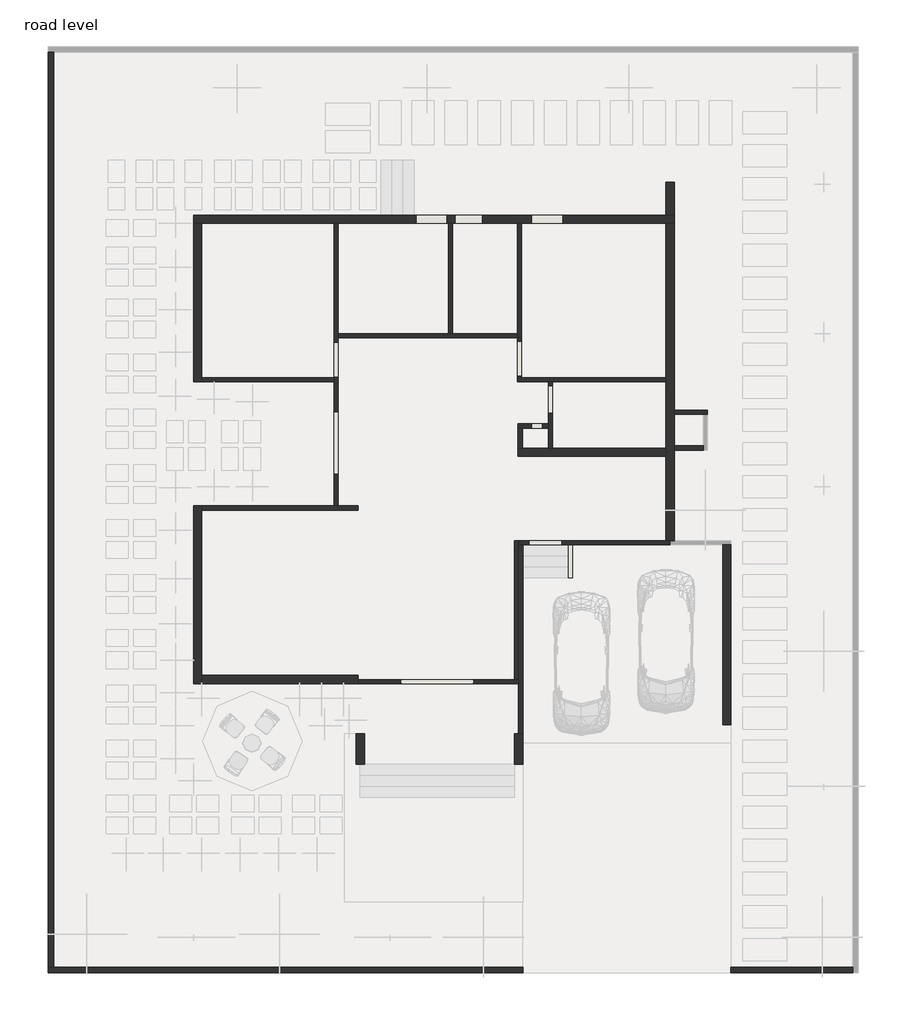
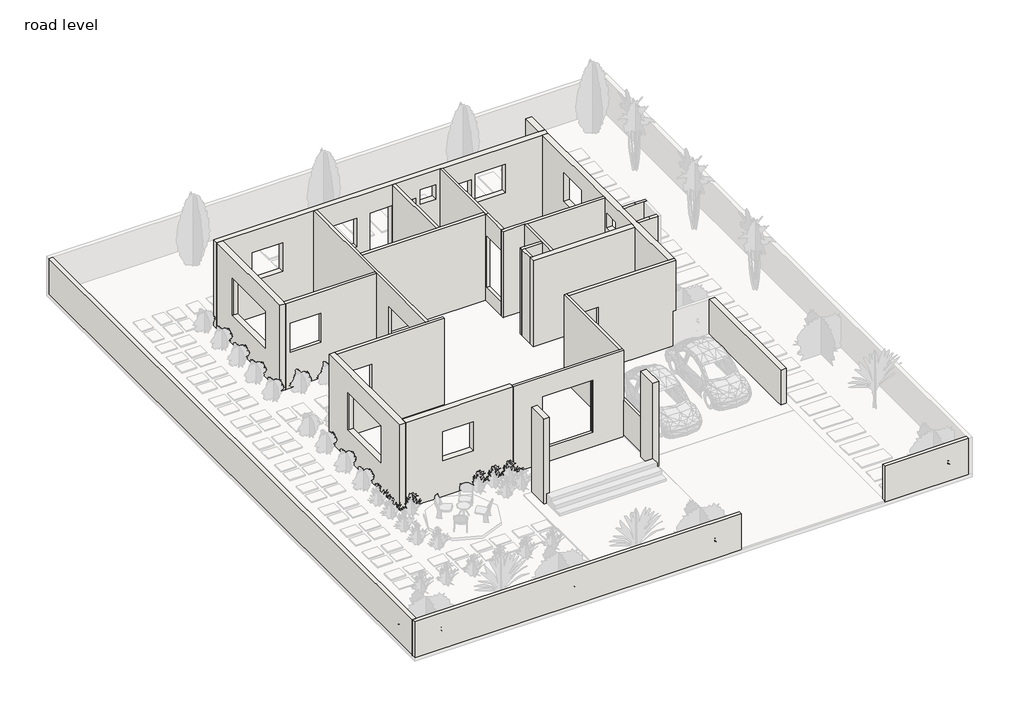
# One storey, part 1 of 3: 31 walls.
"""IFC4 building model written with IfcOpenShell, lengths in millimetres."""

from ifc_helpers import new_model, si_unit, frame, origin, origin_with_axes, place, context, project, spatial, polyline, outline, extrude, faceted_brep, element, save

model = new_model("IFC4")

# Units and contexts
model_context = context("Model", 3, world=origin())
ifc_project = project(units=[si_unit("LENGTHUNIT", "METRE", prefix="MILLI")], contexts=[model_context])

# Site, building, storey
site = spatial("IfcSite", under=ifc_project)
building = spatial("IfcBuilding", under=site)
storey = spatial("IfcBuildingStorey", under=building, Name="road level", Elevation=0.0)

# Walls
placement = place(None, origin())
element("IfcWall", 1, ObjectType="Generic - 4.5\"", at=placement, inside=storey, context=model_context, shape_type="Brep", body=[
    faceted_brep([(-10099.9719122, 10368.3168074, 0.0), (-10099.9719122, 6101.1168074, 0.0), (-10099.9719122, 5986.8168074, 0.0), (-10099.9719122, 2557.8168074, 0.0), (-10099.9719122, 2557.8168074, 3657.6), (-10099.9719122, 5986.8168074, 3657.6), (-10099.9719122, 6101.1168074, 3657.6), (-10099.9719122, 10368.3168074, 3657.6), (-10099.9719122, 6120.1668074, 609.6), (-10099.9719122, 7085.3668074, 609.6), (-10099.9719122, 7085.3668074, 2768.6), (-10099.9719122, 6120.1668074, 2768.6), (-10099.9719122, 5154.9668074, 2743.2), (-10099.9719122, 3427.7668074, 2743.2), (-10099.9719122, 3427.7668074, 609.6), (-10099.9719122, 5154.9668074, 609.6), (-9985.6719122, 10368.3168074, 0.0), (-9985.6719122, 10368.3168074, 3657.6), (-9985.6719122, 7320.3168074, 3657.6), (-9985.6719122, 7206.0168074, 3657.6), (-9985.6719122, 2557.8168074, 3657.6), (-9985.6719122, 2557.8168074, 0.0), (-9985.6719122, 7206.0168074, 0.0), (-9985.6719122, 7320.3168074, 0.0), (-9985.6719122, 6120.1668074, 609.6), (-9985.6719122, 6120.1668074, 2768.6), (-9985.6719122, 7085.3668074, 2768.6), (-9985.6719122, 7085.3668074, 609.6), (-9985.6719122, 5154.9668074, 2743.2), (-9985.6719122, 5154.9668074, 609.6), (-9985.6719122, 3427.7668074, 609.6), (-9985.6719122, 3427.7668074, 2743.2)], [[[0, 1, 2, 3, 4, 5, 6, 7], [8, 9, 10, 11], [12, 13, 14, 15]], [[16, 17, 18, 19, 20, 21, 22, 23], [24, 25, 26, 27], [28, 29, 30, 31]], [[3, 2, 1, 0, 16, 23, 22, 21]], [[0, 7, 17, 16]], [[4, 3, 21, 20]], [[25, 24, 8, 11]], [[26, 25, 11, 10]], [[27, 26, 10, 9]], [[24, 27, 9, 8]], [[29, 28, 12, 15]], [[30, 29, 15, 14]], [[31, 30, 14, 13]], [[28, 31, 13, 12]], [[7, 6, 5, 4, 20, 19, 18, 17]]]),
])
element("IfcWall", 2, ObjectType="Generic - 4.5\"", at=placement, inside=storey, context=model_context, shape_type="SweptSolid", body=[
    extrude(outline(polyline([(0.0, -10099.9719122), (3657.6, -10099.9719122), (3657.6, -13757.5719122), (0.0, -13757.5719122), (0.0, -10099.9719122)]), holes=[polyline([(2743.2, -13567.0719122), (2743.2, -12347.8719122), (1524.0, -12347.8719122), (1524.0, -13567.0719122), (2743.2, -13567.0719122)])]), frame((0.0, 5986.8168074, 0.0), z_axis=(0.0, 1.0, 0.0), x_axis=(0.0, 0.0, 1.0)), (0.0, 0.0, 1.0), 114.3),
])
element("IfcWall", 3, ObjectType="Generic - 4.5\"", at=placement, inside=storey, context=model_context, shape_type="Brep", body=[
    faceted_brep([(-5023.1469122, 10368.3168074, 0.0), (-5023.1469122, 7320.3168074, 0.0), (-5023.1469122, 7206.0168074, 0.0), (-5023.1469122, 7206.0168074, 3657.6), (-5023.1469122, 7320.3168074, 3657.6), (-5023.1469122, 10368.3168074, 3657.6), (-4908.8469122, 10368.3168074, 0.0), (-4908.8469122, 10368.3168074, 3657.6), (-4908.8469122, 7206.0168074, 3657.6), (-4908.8469122, 7206.0168074, 0.0)], [[[0, 1, 2, 3, 4, 5]], [[6, 7, 8, 9]], [[2, 1, 0, 6, 9]], [[0, 5, 7, 6]], [[3, 2, 9, 8]], [[5, 4, 3, 8, 7]]]),
])
element("IfcWall", 4, ObjectType="Generic - 4.5\"", at=placement, inside=storey, context=model_context, shape_type="Brep", body=[
    faceted_brep([(-5023.1469122, 7320.3168074, 0.0), (-6823.3719122, 7320.3168074, 0.0), (-6937.6719122, 7320.3168074, 0.0), (-9985.6719122, 7320.3168074, 0.0), (-9985.6719122, 7320.3168074, 3657.6), (-6937.6719122, 7320.3168074, 3657.6), (-6823.3719122, 7320.3168074, 3657.6), (-5023.1469122, 7320.3168074, 3657.6), (-5023.1469122, 7206.0168074, 0.0), (-5023.1469122, 7206.0168074, 3657.6), (-9985.6719122, 7206.0168074, 3657.6), (-9985.6719122, 7206.0168074, 0.0)], [[[0, 1, 2, 3, 4, 5, 6, 7]], [[8, 9, 10, 11]], [[3, 2, 1, 0, 8, 11]], [[0, 7, 9, 8]], [[4, 3, 11, 10]], [[7, 6, 5, 4, 10, 9]]]),
])
element("IfcWall", 5, ObjectType="Generic - 4.5\"", at=placement, inside=storey, context=model_context, shape_type="SweptSolid", body=[
    extrude(outline(polyline([(-6937.6719122, 7320.3168074), (-6937.6719122, 10368.3168074), (-6823.3719122, 10368.3168074), (-6823.3719122, 7320.3168074), (-6937.6719122, 7320.3168074)])), origin_with_axes(), (0.0, 0.0, 1.0), 3657.6),
])
element("IfcWall", 6, ObjectType="Generic - 4.5\"", at=placement, inside=storey, context=model_context, shape_type="Brep", body=[
    faceted_brep([(-917.8719122, 6101.1168074, 0.0), (-4908.8469122, 6101.1168074, 0.0), (-5023.1469122, 6101.1168074, 0.0), (-5023.1469122, 6101.1168074, 3657.6), (-4908.8469122, 6101.1168074, 3657.6), (-917.8719122, 6101.1168074, 3657.6), (-917.8719122, 5986.8168074, 0.0), (-917.8719122, 5986.8168074, 3657.6), (-4054.7719122, 5986.8168074, 3657.6), (-4169.0719122, 5986.8168074, 3657.6), (-5023.1469122, 5986.8168074, 3657.6), (-5023.1469122, 5986.8168074, 0.0), (-4169.0719122, 5986.8168074, 0.0), (-4054.7719122, 5986.8168074, 0.0)], [[[0, 1, 2, 3, 4, 5]], [[6, 7, 8, 9, 10, 11, 12, 13]], [[2, 1, 0, 6, 13, 12, 11]], [[3, 2, 11, 10]], [[0, 5, 7, 6]], [[5, 4, 3, 10, 9, 8, 7]]]),
])
element("IfcWall", 7, ObjectType="Generic - 4.5\"", at=placement, inside=storey, context=model_context, shape_type="SweptSolid", body=[
    extrude(outline(polyline([(6101.1168074, 0.0), (6101.1168074, 3657.6), (7206.0168074, 3657.6), (7206.0168074, 0.0), (6101.1168074, 0.0)]), holes=[polyline([(6142.3918074, 609.6), (7107.5918074, 609.6), (7107.5918074, 2768.6), (6142.3918074, 2768.6), (6142.3918074, 609.6)])]), frame((-5023.1469122, 0.0, 0.0), z_axis=(1.0, 0.0, 0.0), x_axis=(0.0, 1.0, 0.0)), (0.0, 0.0, 1.0), 114.3),
])
element("IfcWall", 8, ObjectType="Generic - 4.5\"", at=placement, inside=storey, context=model_context, shape_type="Brep", body=[
    faceted_brep([(-13757.5719122, 2443.5168074, 0.0), (-9433.2219122, 2443.5168074, 0.0), (-9433.2219122, 2443.5168074, 3657.6), (-13757.5719122, 2443.5168074, 3657.6), (-12347.8719122, 2443.5168074, 2743.2), (-12347.8719122, 2443.5168074, 1524.0), (-13567.0719122, 2443.5168074, 1524.0), (-13567.0719122, 2443.5168074, 2743.2), (-13757.5719122, 2557.8168074, 0.0), (-13757.5719122, 2557.8168074, 3657.6), (-10099.9719122, 2557.8168074, 3657.6), (-9985.6719122, 2557.8168074, 3657.6), (-9433.2219122, 2557.8168074, 3657.6), (-9433.2219122, 2557.8168074, 0.0), (-9985.6719122, 2557.8168074, 0.0), (-10099.9719122, 2557.8168074, 0.0), (-12347.8719122, 2557.8168074, 2743.2), (-13567.0719122, 2557.8168074, 2743.2), (-13567.0719122, 2557.8168074, 1524.0), (-12347.8719122, 2557.8168074, 1524.0)], [[[0, 1, 2, 3], [4, 5, 6, 7]], [[8, 9, 10, 11, 12, 13, 14, 15], [16, 17, 18, 19]], [[1, 0, 8, 15, 14, 13]], [[2, 1, 13, 12]], [[0, 3, 9, 8]], [[5, 4, 16, 19]], [[6, 5, 19, 18]], [[7, 6, 18, 17]], [[4, 7, 17, 16]], [[3, 2, 12, 11, 10, 9]]]),
])
element("IfcWall", 9, ObjectType="Generic - 4.5\"", at=placement, inside=storey, context=model_context, shape_type="Brep", body=[
    faceted_brep([(-9433.2219122, -2357.0831926, 0.0), (-4994.5719122, -2357.0831926, 0.0), (-4994.5719122, -2357.0831926, 3657.6), (-9433.2219122, -2357.0831926, 3657.6), (-8242.4719122, -2357.0831926, 2818.6), (-6242.4719122, -2357.0831926, 2818.6), (-6242.4719122, -2357.0831926, 609.6), (-8242.4719122, -2357.0831926, 609.6), (-4994.5719122, -2242.7831926, 0.0), (-5108.8719122, -2242.7831926, 0.0), (-9433.2219122, -2242.7831926, 0.0), (-9433.2219122, -2242.7831926, 3657.6), (-5108.8719122, -2242.7831926, 3657.6), (-4994.5719122, -2242.7831926, 3657.6), (-6242.4719122, -2242.7831926, 2818.6), (-8242.4719122, -2242.7831926, 2818.6), (-8242.4719122, -2242.7831926, 609.6), (-6242.4719122, -2242.7831926, 609.6), (-6242.4719122, -2262.7831926, 2818.6), (-8242.4719122, -2262.7831926, 2818.6), (-8242.4719122, -2332.7831926, 2818.6), (-6242.4719122, -2332.7831926, 2818.6), (-6242.4719122, -2332.7831926, 609.6), (-6227.4719122, -2332.7831926, 609.6), (-6227.4719122, -2262.7831926, 609.6), (-6242.4719122, -2262.7831926, 609.6), (-8242.4719122, -2262.7831926, 609.6), (-8257.4719122, -2262.7831926, 609.6), (-8257.4719122, -2332.7831926, 609.6), (-8242.4719122, -2332.7831926, 609.6), (-8257.4719122, -2332.7831926, 2833.6), (-6227.4719122, -2332.7831926, 2833.6), (-6227.4719122, -2262.7831926, 2833.6), (-8257.4719122, -2262.7831926, 2833.6)], [[[0, 1, 2, 3], [4, 5, 6, 7]], [[8, 9, 10, 11, 12, 13], [14, 15, 16, 17]], [[1, 0, 10, 9, 8]], [[0, 3, 11, 10]], [[2, 1, 8, 13]], [[18, 19, 15, 14]], [[20, 21, 5, 4]], [[22, 23, 24, 25, 17, 16, 26, 27, 28, 29, 7, 6]], [[29, 20, 4, 7]], [[21, 22, 6, 5]], [[21, 20, 29, 28, 30, 31, 23, 22]], [[24, 23, 31, 32]], [[19, 18, 25, 24, 32, 33, 27, 26]], [[25, 18, 14, 17]], [[19, 26, 16, 15]], [[28, 27, 33, 30]], [[31, 30, 33, 32]], [[3, 2, 13, 12, 11]]]),
])
element("IfcWall", 10, ObjectType="Generic - 4.5\"", at=placement, inside=storey, context=model_context, shape_type="Brep", body=[
    faceted_brep([(-4994.5719122, -2242.7831926, 0.0), (-4994.5719122, 1481.4918074, 0.0), (-4994.5719122, 1595.7918074, 0.0), (-4994.5719122, 1595.7918074, 3657.6), (-4994.5719122, 1481.4918074, 3657.6), (-4994.5719122, -2242.7831926, 3657.6), (-5108.8719122, -2242.7831926, 0.0), (-5108.8719122, -2242.7831926, 3657.6), (-5108.8719122, 1595.7918074, 3657.6), (-5108.8719122, 1595.7918074, 0.0)], [[[0, 1, 2, 3, 4, 5]], [[6, 7, 8, 9]], [[2, 1, 0, 6, 9]], [[0, 5, 7, 6]], [[3, 2, 9, 8]], [[5, 4, 3, 8, 7]]]),
])
element("IfcWall", 11, ObjectType="Generic - 4.5\"", at=placement, inside=storey, context=model_context, shape_type="Brep", body=[
    faceted_brep([(-4994.5719122, 1481.4918074, 0.0), (-4993.7781622, 1481.4918074, 0.0), (-4879.4781622, 1481.4918074, 0.0), (-3616.6219122, 1481.4918074, 0.0), (-3502.3219122, 1481.4918074, 0.0), (-803.5719122, 1481.4918074, 0.0), (-803.5719122, 1481.4918074, 1524.0), (-689.2719122, 1481.4918074, 1524.0), (-689.2719122, 1481.4918074, 3657.6), (-4994.5719122, 1481.4918074, 3657.6), (-4708.0281622, 1481.4918074, 2743.2), (-3793.6281622, 1481.4918074, 2743.2), (-3793.6281622, 1481.4918074, 609.6), (-4708.0281622, 1481.4918074, 609.6), (-4994.5719122, 1595.7918074, 0.0), (-4994.5719122, 1595.7918074, 3657.6), (-917.8719122, 1595.7918074, 3657.6), (-689.2719122, 1595.7918074, 3657.6), (-689.2719122, 1595.7918074, 1524.0), (-803.5719122, 1595.7918074, 1524.0), (-803.5719122, 1595.7918074, 0.0), (-917.8719122, 1595.7918074, 0.0), (-4708.0281622, 1595.7918074, 2743.2), (-4708.0281622, 1595.7918074, 609.6), (-3793.6281622, 1595.7918074, 609.6), (-3793.6281622, 1595.7918074, 2743.2)], [[[0, 1, 2, 3, 4, 5, 6, 7, 8, 9], [10, 11, 12, 13]], [[14, 15, 16, 17, 18, 19, 20, 21], [22, 23, 24, 25]], [[5, 4, 3, 2, 1, 0, 14, 21, 20]], [[0, 9, 15, 14]], [[6, 5, 20, 19]], [[18, 7, 6, 19]], [[8, 7, 18, 17]], [[23, 22, 10, 13]], [[24, 23, 13, 12]], [[25, 24, 12, 11]], [[22, 25, 11, 10]], [[9, 8, 17, 16, 15]]]),
])
element("IfcWall", 12, ObjectType="Generic - 4.5\"", at=placement, inside=storey, context=model_context, shape_type="SweptSolid", body=[
    extrude(outline(polyline([(-4879.4781622, 1481.4918074), (-4879.4781622, -3741.3831926), (-4993.7781622, -3741.3831926), (-4993.7781622, 1481.4918074), (-4879.4781622, 1481.4918074)])), origin_with_axes(), (0.0, 0.0, 1.0), 1524.0),
])
element("IfcWall", 13, ObjectType="Generic - 4.5\"", at=placement, inside=storey, context=model_context, shape_type="SweptSolid", body=[
    extrude(outline(polyline([(-3502.3219122, 1481.4918074), (-3502.3219122, 566.1722231), (-3616.6219122, 566.1722231), (-3616.6219122, 1481.4918074), (-3502.3219122, 1481.4918074)])), origin_with_axes(), (0.0, 0.0, 1.0), 609.6),
])
element("IfcWall", 14, ObjectType="Generic - 4.5\"", at=placement, inside=storey, context=model_context, shape_type="Brep", body=[
    faceted_brep([(-4054.7719122, 4158.0168074, 0.0), (-4054.7719122, 5986.8168074, 0.0), (-4054.7719122, 5986.8168074, 3657.6), (-4054.7719122, 4158.0168074, 3657.6), (-4054.7719122, 5123.2168074, 609.6), (-4054.7719122, 5123.2168074, 2743.2), (-4054.7719122, 5885.2168074, 2743.2), (-4054.7719122, 5885.2168074, 609.6), (-4169.0719122, 4158.0168074, 0.0), (-4169.0719122, 4158.0168074, 3657.6), (-4169.0719122, 4710.4668074, 3657.6), (-4169.0719122, 4824.7668074, 3657.6), (-4169.0719122, 5986.8168074, 3657.6), (-4169.0719122, 5986.8168074, 0.0), (-4169.0719122, 4824.7668074, 0.0), (-4169.0719122, 4710.4668074, 0.0), (-4169.0719122, 5123.2168074, 609.6), (-4169.0719122, 5885.2168074, 609.6), (-4169.0719122, 5885.2168074, 2743.2), (-4169.0719122, 5123.2168074, 2743.2)], [[[0, 1, 2, 3], [4, 5, 6, 7]], [[8, 9, 10, 11, 12, 13, 14, 15], [16, 17, 18, 19]], [[1, 0, 8, 15, 14, 13]], [[2, 1, 13, 12]], [[0, 3, 9, 8]], [[17, 16, 4, 7]], [[18, 17, 7, 6]], [[19, 18, 6, 5]], [[16, 19, 5, 4]], [[3, 2, 12, 11, 10, 9]]]),
])
element("IfcWall", 15, ObjectType="Generic - 4.5\"", at=placement, inside=storey, context=model_context, shape_type="SweptSolid", body=[
    extrude(outline(polyline([(-4892.1918815, 4710.4668074), (-4892.1918815, 4158.0168074), (-5006.4918815, 4158.0168074), (-5006.4918815, 4710.4668074), (-4892.1918815, 4710.4668074)])), origin_with_axes(), (0.0, 0.0, 1.0), 3657.6),
])
element("IfcWall", 16, ObjectType="Generic - 4.5\"", at=placement, inside=storey, context=model_context, shape_type="Brep", body=[
    faceted_brep([(-5006.4918815, 4710.4668074, 0.0), (-4892.1918815, 4710.4668074, 0.0), (-4169.0719122, 4710.4668074, 0.0), (-4169.0719122, 4710.4668074, 3657.6), (-4892.1918815, 4710.4668074, 3657.6), (-5006.4918815, 4710.4668074, 3657.6), (-4334.1719122, 4710.4668074, 609.6), (-4638.9719122, 4710.4668074, 609.6), (-4638.9719122, 4710.4668074, 2438.4), (-4334.1719122, 4710.4668074, 2438.4), (-4169.0719122, 4824.7668074, 0.0), (-5006.4918815, 4824.7668074, 0.0), (-5006.4918815, 4824.7668074, 3657.6), (-4169.0719122, 4824.7668074, 3657.6), (-4638.9719122, 4824.7668074, 609.6), (-4334.1719122, 4824.7668074, 609.6), (-4334.1719122, 4824.7668074, 2438.4), (-4638.9719122, 4824.7668074, 2438.4)], [[[0, 1, 2, 3, 4, 5], [6, 7, 8, 9]], [[10, 11, 12, 13], [14, 15, 16, 17]], [[2, 1, 0, 11, 10]], [[3, 2, 10, 13]], [[0, 5, 12, 11]], [[14, 7, 6, 15]], [[16, 9, 8, 17]], [[7, 14, 17, 8]], [[9, 16, 15, 6]], [[5, 4, 3, 13, 12]]]),
])
element("IfcWall", 17, ObjectType="Generic - 4.5\"", at=placement, inside=storey, context=model_context, shape_type="Brep", body=[
    faceted_brep([(-689.2719122, 5091.4668074, 0.0), (117.1780878, 5091.4668074, 0.0), (231.4780878, 5091.4668074, 0.0), (231.4780878, 5091.4668074, 3657.6), (117.1780878, 5091.4668074, 3657.6), (-193.9719122, 5091.4668074, 3657.6), (-689.2719122, 5091.4668074, 3657.6), (-689.2719122, 5205.7668074, 0.0), (-689.2719122, 5205.7668074, 3657.6), (-193.9719122, 5205.7668074, 3657.6), (231.4780878, 5205.7668074, 3657.6), (231.4780878, 5205.7668074, 0.0)], [[[0, 1, 2, 3, 4, 5, 6]], [[7, 8, 9, 10, 11]], [[2, 1, 0, 7, 11]], [[0, 6, 8, 7]], [[3, 2, 11, 10]], [[5, 4, 3, 10, 9]], [[6, 5, 9, 8]]]),
])
element("IfcWall", 18, ObjectType="Generic - 4.5\"", at=placement, inside=storey, context=model_context, shape_type="SweptSolid", body=[
    extrude(outline(polyline([(0.0, 117.1780878), (3657.6, 117.1780878), (3657.6, -193.9719122), (3657.6, -689.2719122), (0.0, -689.2719122), (0.0, 117.1780878)])), frame((0.0, 4100.8668074, 0.0), z_axis=(0.0, 1.0, 0.0), x_axis=(0.0, 0.0, 1.0)), (0.0, 0.0, 1.0), 114.3),
])
element("IfcWall", 19, ObjectType="Generic - 6\"", at=placement, inside=storey, context=model_context, shape_type="SweptSolid", body=[
    extrude(outline(polyline([(879.1423374, -10192.2627683), (4247.9423756, -10192.2627683), (4247.9423756, -10344.6627683), (879.1423374, -10344.6627683), (879.1423374, -10192.2627683)])), origin_with_axes(), (0.0, 0.0, 1.0), 1524.0),
])
element("IfcWall", 20, ObjectType="Generic - 6\"", at=placement, inside=storey, context=model_context, shape_type="SweptSolid", body=[
    extrude(outline(polyline([(-17850.0576244, 15106.1372317), (-17850.0576244, -10192.2627683), (-18002.4576244, -10192.2627683), (-18002.4576244, 15106.1372317), (-17850.0576244, 15106.1372317)])), origin_with_axes(), (0.0, 0.0, 1.0), 1524.0),
])
element("IfcWall", 21, ObjectType="Generic - 6\"", at=placement, inside=storey, context=model_context, shape_type="Brep", body=[
    faceted_brep([(-4879.6043753, -10192.2627683, 0.0), (-17850.0576244, -10192.2627683, 0.0), (-18002.4576244, -10192.2627683, 0.0), (-18002.4576244, -10192.2627683, 1524.0), (-17850.0576244, -10192.2627683, 1524.0), (-4879.6043753, -10192.2627683, 1524.0), (-4879.6043753, -10344.6627683, 0.0), (-4879.6043753, -10344.6627683, 1524.0), (-18002.4576244, -10344.6627683, 1524.0), (-18002.4576244, -10344.6627683, 0.0)], [[[0, 1, 2, 3, 4, 5]], [[6, 7, 8, 9]], [[2, 1, 0, 6, 9]], [[5, 4, 3, 8, 7]], [[0, 5, 7, 6]], [[3, 2, 9, 8]]]),
])
element("IfcWall", 22, ObjectType="Generic - 9\"", at=placement, inside=storey, context=model_context, shape_type="Brep", body=[
    faceted_brep([(-13986.1719122, 10368.3168074, 0.0), (-13757.5719122, 10368.3168074, 0.0), (-10099.9719122, 10368.3168074, 0.0), (-9985.6719122, 10368.3168074, 0.0), (-6937.6719122, 10368.3168074, 0.0), (-6823.3719122, 10368.3168074, 0.0), (-5023.1469122, 10368.3168074, 0.0), (-4908.8469122, 10368.3168074, 0.0), (-917.8719122, 10368.3168074, 0.0), (-689.2719122, 10368.3168074, 0.0), (-689.2719122, 10368.3168074, 3657.6), (-917.8719122, 10368.3168074, 3657.6), (-4908.8469122, 10368.3168074, 3657.6), (-5023.1469122, 10368.3168074, 3657.6), (-6823.3719122, 10368.3168074, 3657.6), (-6937.6719122, 10368.3168074, 3657.6), (-9985.6719122, 10368.3168074, 3657.6), (-10099.9719122, 10368.3168074, 3657.6), (-13757.5719122, 10368.3168074, 3657.6), (-13986.1719122, 10368.3168074, 3657.6), (-6969.4219122, 10368.3168074, 609.6), (-7833.0219122, 10368.3168074, 609.6), (-7833.0219122, 10368.3168074, 2768.6), (-6969.4219122, 10368.3168074, 2768.6), (-4635.7969122, 10368.3168074, 609.6), (-4635.7969122, 10368.3168074, 2768.6), (-3772.1969122, 10368.3168074, 2768.6), (-3772.1969122, 10368.3168074, 609.6), (-5991.5219122, 10368.3168074, 609.6), (-6753.5219122, 10368.3168074, 609.6), (-6753.5219122, 10368.3168074, 2743.2), (-5991.5219122, 10368.3168074, 2743.2), (-5810.5469122, 10368.3168074, 3048.0), (-5200.9469122, 10368.3168074, 3048.0), (-5200.9469122, 10368.3168074, 2438.4), (-5810.5469122, 10368.3168074, 2438.4), (-8366.4219122, 10368.3168074, 2743.2), (-8366.4219122, 10368.3168074, 1524.0), (-9585.6219122, 10368.3168074, 1524.0), (-9585.6219122, 10368.3168074, 2743.2), (-11347.7469122, 10368.3168074, 2743.2), (-11347.7469122, 10368.3168074, 1524.0), (-12566.9469122, 10368.3168074, 1524.0), (-12566.9469122, 10368.3168074, 2743.2), (-2400.5969122, 10368.3168074, 2946.4), (-2400.5969122, 10368.3168074, 1727.2), (-3619.7969122, 10368.3168074, 1727.2), (-3619.7969122, 10368.3168074, 2946.4), (-13986.1719122, 10596.9168074, 0.0), (-13986.1719122, 10596.9168074, 3657.6), (-5137.4469122, 10596.9168074, 3657.6), (-4908.8469122, 10596.9168074, 3657.6), (-917.8719122, 10596.9168074, 3657.6), (-689.2719122, 10596.9168074, 3657.6), (-689.2719122, 10596.9168074, 0.0), (-917.8719122, 10596.9168074, 0.0), (-6969.4219122, 10596.9168074, 609.6), (-6969.4219122, 10596.9168074, 2768.6), (-7833.0219122, 10596.9168074, 2768.6), (-7833.0219122, 10596.9168074, 609.6), (-4635.7969122, 10596.9168074, 609.6), (-3772.1969122, 10596.9168074, 609.6), (-3772.1969122, 10596.9168074, 2768.6), (-4635.7969122, 10596.9168074, 2768.6), (-5991.5219122, 10596.9168074, 609.6), (-5991.5219122, 10596.9168074, 2743.2), (-6753.5219122, 10596.9168074, 2743.2), (-6753.5219122, 10596.9168074, 609.6), (-5810.5469122, 10596.9168074, 3048.0), (-5810.5469122, 10596.9168074, 2438.4), (-5200.9469122, 10596.9168074, 2438.4), (-5200.9469122, 10596.9168074, 3048.0), (-8366.4219122, 10596.9168074, 2743.2), (-9585.6219122, 10596.9168074, 2743.2), (-9585.6219122, 10596.9168074, 1524.0), (-8366.4219122, 10596.9168074, 1524.0), (-11347.7469122, 10596.9168074, 2743.2), (-12566.9469122, 10596.9168074, 2743.2), (-12566.9469122, 10596.9168074, 1524.0), (-11347.7469122, 10596.9168074, 1524.0), (-2400.5969122, 10596.9168074, 2946.4), (-3619.7969122, 10596.9168074, 2946.4), (-3619.7969122, 10596.9168074, 1727.2), (-2400.5969122, 10596.9168074, 1727.2)], [[[0, 1, 2, 3, 4, 5, 6, 7, 8, 9, 10, 11, 12, 13, 14, 15, 16, 17, 18, 19], [20, 21, 22, 23], [24, 25, 26, 27], [28, 29, 30, 31], [32, 33, 34, 35], [36, 37, 38, 39], [40, 41, 42, 43], [44, 45, 46, 47]], [[48, 49, 50, 51, 52, 53, 54, 55], [56, 57, 58, 59], [60, 61, 62, 63], [64, 65, 66, 67], [68, 69, 70, 71], [72, 73, 74, 75], [76, 77, 78, 79], [80, 81, 82, 83]], [[9, 8, 7, 6, 5, 4, 3, 2, 1, 0, 48, 55, 54]], [[0, 19, 49, 48]], [[10, 9, 54, 53]], [[57, 56, 20, 23]], [[58, 57, 23, 22]], [[59, 58, 22, 21]], [[56, 59, 21, 20]], [[25, 24, 60, 63]], [[26, 25, 63, 62]], [[27, 26, 62, 61]], [[24, 27, 61, 60]], [[29, 28, 64, 67]], [[30, 29, 67, 66]], [[31, 30, 66, 65]], [[28, 31, 65, 64]], [[69, 68, 32, 35]], [[70, 69, 35, 34]], [[71, 70, 34, 33]], [[68, 71, 33, 32]], [[37, 36, 72, 75]], [[38, 37, 75, 74]], [[39, 38, 74, 73]], [[36, 39, 73, 72]], [[41, 40, 76, 79]], [[42, 41, 79, 78]], [[43, 42, 78, 77]], [[40, 43, 77, 76]], [[45, 44, 80, 83]], [[46, 45, 83, 82]], [[47, 46, 82, 81]], [[44, 47, 81, 80]], [[19, 18, 17, 16, 15, 14, 13, 12, 11, 10, 53, 52, 51, 50, 49]]]),
])
element("IfcWall", 23, ObjectType="Generic - 9\"", at=placement, inside=storey, context=model_context, shape_type="Brep", body=[
    faceted_brep([(-13986.1719122, 10368.3168074, 0.0), (-13986.1719122, 5986.8168074, 0.0), (-13986.1719122, 5986.8168074, 3657.6), (-13986.1719122, 10368.3168074, 3657.6), (-13986.1719122, 9316.8211326, 2794.0), (-13986.1719122, 7006.5624822, 2794.0), (-13986.1719122, 7006.5624822, 1219.2), (-13986.1719122, 9316.8211326, 1219.2), (-13757.5719122, 10368.3168074, 0.0), (-13757.5719122, 10368.3168074, 3657.6), (-13757.5719122, 6101.1168074, 3657.6), (-13757.5719122, 5986.8168074, 3657.6), (-13757.5719122, 5986.8168074, 0.0), (-13757.5719122, 6101.1168074, 0.0), (-13757.5719122, 7018.6918074, 2794.0), (-13757.5719122, 9304.6918074, 2794.0), (-13757.5719122, 9304.6918074, 1219.2), (-13757.5719122, 7018.6918074, 1219.2), (-13917.3830906, 7018.6918074, 2794.0), (-13917.3830906, 9304.6918074, 2794.0), (-13917.3830906, 7018.6918074, 1219.2), (-13917.3830906, 9304.6918074, 1219.2)], [[[0, 1, 2, 3], [4, 5, 6, 7]], [[8, 9, 10, 11, 12, 13], [14, 15, 16, 17]], [[1, 0, 8, 13, 12]], [[0, 3, 9, 8]], [[2, 1, 12, 11]], [[18, 5, 4, 19, 15, 14]], [[20, 17, 16, 21, 7, 6]], [[18, 14, 17, 20]], [[15, 19, 21, 16]], [[19, 4, 7, 21]], [[5, 18, 20, 6]], [[3, 2, 11, 10, 9]]]),
])
element("IfcWall", 24, ObjectType="Generic - 9\"", at=placement, inside=storey, context=model_context, shape_type="Brep", body=[
    faceted_brep([(-9433.2219122, -2128.4831926, 0.0), (-13757.5719122, -2128.4831926, 0.0), (-13757.5719122, -2128.4831926, 3657.6), (-9433.2219122, -2128.4831926, 3657.6), (-12262.1469122, -2128.4831926, 2743.2), (-12262.1469122, -2128.4831926, 1524.0), (-11042.9469122, -2128.4831926, 1524.0), (-11042.9469122, -2128.4831926, 2743.2), (-9433.2219122, -2357.0831926, 0.0), (-9433.2219122, -2357.0831926, 3657.6), (-13757.5719122, -2357.0831926, 3657.6), (-13757.5719122, -2357.0831926, 0.0), (-12262.1469122, -2357.0831926, 2743.2), (-11042.9469122, -2357.0831926, 2743.2), (-11042.9469122, -2357.0831926, 1524.0), (-12262.1469122, -2357.0831926, 1524.0), (-9433.2219122, -2242.7831926, 0.0), (-9433.2219122, -2242.7831926, 3657.6)], [[[0, 1, 2, 3], [4, 5, 6, 7]], [[8, 9, 10, 11], [12, 13, 14, 15]], [[1, 0, 16, 8, 11]], [[0, 3, 17, 9, 8, 16]], [[2, 1, 11, 10]], [[5, 4, 12, 15]], [[6, 5, 15, 14]], [[7, 6, 14, 13]], [[4, 7, 13, 12]], [[3, 2, 10, 9, 17]]]),
])
element("IfcWall", 25, ObjectType="Generic - 9\"", at=placement, inside=storey, context=model_context, shape_type="SweptSolid", body=[
    extrude(outline(polyline([(650.5780878, -3492.1743478), (650.5780878, 1481.4918074), (879.1780878, 1481.4918074), (879.1780878, -3492.1743478), (650.5780878, -3492.1743478)])), origin_with_axes(), (0.0, 0.0, 1.0), 1524.0),
])
element("IfcWall", 26, ObjectType="Generic - 9\"", at=placement, inside=storey, context=model_context, shape_type="Brep", body=[
    faceted_brep([(-917.8719122, 10368.3168074, 0.0), (-917.8719122, 6101.1168074, 0.0), (-917.8719122, 5986.8168074, 0.0), (-917.8719122, 4158.0168074, 0.0), (-917.8719122, 3929.4168074, 0.0), (-917.8719122, 1595.7918074, 0.0), (-917.8719122, 1595.7918074, 3657.6), (-917.8719122, 3929.4168074, 3657.6), (-917.8719122, 4158.0168074, 3657.6), (-917.8719122, 5986.8168074, 3657.6), (-917.8719122, 6101.1168074, 3657.6), (-917.8719122, 10368.3168074, 3657.6), (-917.8719122, 5891.5668074, 3048.0), (-917.8719122, 5281.9668074, 3048.0), (-917.8719122, 5281.9668074, 2438.4), (-917.8719122, 5891.5668074, 2438.4), (-917.8719122, 7653.6918074, 2971.8), (-917.8719122, 7653.6918074, 1752.6), (-917.8719122, 8872.8918074, 1752.6), (-917.8719122, 8872.8918074, 2971.8), (-689.2719122, 10368.3168074, 0.0), (-689.2719122, 10368.3168074, 3657.6), (-689.2719122, 5205.7668074, 3657.6), (-689.2719122, 5091.4668074, 3657.6), (-689.2719122, 4215.1668074, 3657.6), (-689.2719122, 4100.8668074, 3657.6), (-689.2719122, 1595.7918074, 3657.6), (-689.2719122, 1595.7918074, 1524.0), (-689.2719122, 1595.7918074, 0.0), (-689.2719122, 4100.8668074, 0.0), (-689.2719122, 4215.1668074, 0.0), (-689.2719122, 5091.4668074, 0.0), (-689.2719122, 5205.7668074, 0.0), (-689.2719122, 5891.5668074, 3048.0), (-689.2719122, 5891.5668074, 2438.4), (-689.2719122, 5281.9668074, 2438.4), (-689.2719122, 5281.9668074, 3048.0), (-689.2719122, 7653.6918074, 2971.8), (-689.2719122, 8872.8918074, 2971.8), (-689.2719122, 8872.8918074, 1752.6), (-689.2719122, 7653.6918074, 1752.6), (-803.5719122, 1595.7918074, 0.0)], [[[0, 1, 2, 3, 4, 5, 6, 7, 8, 9, 10, 11], [12, 13, 14, 15], [16, 17, 18, 19]], [[20, 21, 22, 23, 24, 25, 26, 27, 28, 29, 30, 31, 32], [33, 34, 35, 36], [37, 38, 39, 40]], [[5, 4, 3, 2, 1, 0, 20, 32, 31, 30, 29, 28, 41]], [[0, 11, 21, 20]], [[5, 41, 28, 27, 26, 6]], [[34, 33, 12, 15]], [[35, 34, 15, 14]], [[36, 35, 14, 13]], [[33, 36, 13, 12]], [[17, 16, 37, 40]], [[18, 17, 40, 39]], [[19, 18, 39, 38]], [[16, 19, 38, 37]], [[11, 10, 9, 8, 7, 6, 26, 25, 24, 23, 22, 21]]]),
])
element("IfcWall", 27, ObjectType="Generic - 9\"", at=placement, inside=storey, context=model_context, shape_type="Brep", body=[
    faceted_brep([(-917.8719122, 4158.0168074, 0.0), (-4054.7719122, 4158.0168074, 0.0), (-4169.0719122, 4158.0168074, 0.0), (-4892.1918815, 4158.0168074, 0.0), (-5006.4918815, 4158.0168074, 0.0), (-5006.4918815, 4158.0168074, 3657.6), (-4892.1918815, 4158.0168074, 3657.6), (-4169.0719122, 4158.0168074, 3657.6), (-4054.7719122, 4158.0168074, 3657.6), (-917.8719122, 4158.0168074, 3657.6), (-917.8719122, 3929.4168074, 0.0), (-917.8719122, 3929.4168074, 3657.6), (-5006.4918815, 3929.4168074, 3657.6), (-5006.4918815, 3929.4168074, 0.0)], [[[0, 1, 2, 3, 4, 5, 6, 7, 8, 9]], [[10, 11, 12, 13]], [[4, 3, 2, 1, 0, 10, 13]], [[0, 9, 11, 10]], [[5, 4, 13, 12]], [[9, 8, 7, 6, 5, 12, 11]]]),
])
element("IfcWall", 28, ObjectType="Generic - 9\"", at=placement, inside=storey, context=model_context, shape_type="SweptSolid", body=[
    extrude(outline(polyline([(-9490.3719122, -4585.9331926), (-9490.3719122, -3741.3831926), (-9261.7719122, -3741.3831926), (-9261.7719122, -4585.9331926), (-9490.3719122, -4585.9331926)])), origin_with_axes(), (0.0, 0.0, 1.0), 3657.6),
])
element("IfcWall", 29, ObjectType="Generic - 9\"", at=placement, inside=storey, context=model_context, shape_type="Brep", body=[
    faceted_brep([(-5108.0781622, -3741.3831926, 0.0), (-5108.0781622, -4585.9331926, 0.0), (-5108.0781622, -4585.9331926, 3657.6), (-5108.0781622, -3741.3831926, 3657.6), (-4879.4781622, -3741.3831926, 0.0), (-4879.4781622, -3741.3831926, 1524.0), (-4879.4781622, -3741.3831926, 3657.6), (-4879.4781622, -4585.9331926, 3657.6), (-4879.4781622, -4585.9331926, 0.0), (-4993.7781622, -3741.3831926, 0.0)], [[[0, 1, 2, 3]], [[4, 5, 6, 7, 8]], [[1, 0, 9, 4, 8]], [[2, 1, 8, 7]], [[0, 3, 6, 5, 4, 9]], [[3, 2, 7, 6]]]),
])
element("IfcWall", 30, ObjectType="Generic - 9\"", at=placement, inside=storey, context=model_context, shape_type="SweptSolid", body=[
    extrude(outline(polyline([(-689.2719122, 11511.3168074), (-689.2719122, 10596.9168074), (-917.8719122, 10596.9168074), (-917.8719122, 11511.3168074), (-689.2719122, 11511.3168074)])), origin_with_axes(), (0.0, 0.0, 1.0), 3657.6),
])
element("IfcWall", 31, ObjectType="Generic - 9\"", at=placement, inside=storey, context=model_context, shape_type="Brep", body=[
    faceted_brep([(-13986.1719122, 2557.8168074, 0.0), (-13986.1719122, -2357.0831926, 0.0), (-13986.1719122, -2357.0831926, 3657.6), (-13986.1719122, 2557.8168074, 3657.6), (-13986.1719122, 1284.0711326, 2794.0), (-13986.1719122, -1026.1875178, 2794.0), (-13986.1719122, -1026.1875178, 1219.2), (-13986.1719122, 1284.0711326, 1219.2), (-13757.5719122, 2557.8168074, 0.0), (-13757.5719122, 2557.8168074, 3657.6), (-13757.5719122, 2443.5168074, 3657.6), (-13757.5719122, -2128.4831926, 3657.6), (-13757.5719122, -2357.0831926, 3657.6), (-13757.5719122, -2357.0831926, 0.0), (-13757.5719122, -2128.4831926, 0.0), (-13757.5719122, 2443.5168074, 0.0), (-13757.5719122, -1014.0581926, 2794.0), (-13757.5719122, 1271.9418074, 2794.0), (-13757.5719122, 1271.9418074, 1219.2), (-13757.5719122, -1014.0581926, 1219.2), (-13917.3830906, -1014.0581926, 2794.0), (-13917.3830906, 1271.9418074, 2794.0), (-13917.3830906, -1014.0581926, 1219.2), (-13917.3830906, 1271.9418074, 1219.2)], [[[0, 1, 2, 3], [4, 5, 6, 7]], [[8, 9, 10, 11, 12, 13, 14, 15], [16, 17, 18, 19]], [[1, 0, 8, 15, 14, 13]], [[0, 3, 9, 8]], [[2, 1, 13, 12]], [[20, 5, 4, 21, 17, 16]], [[22, 19, 18, 23, 7, 6]], [[20, 16, 19, 22]], [[17, 21, 23, 18]], [[21, 4, 7, 23]], [[5, 20, 22, 6]], [[3, 2, 12, 11, 10, 9]]]),
])

save(model, "model.ifc")

# Revit data of these elements
# Type "Generic - 4.5\""
#   Assembly Code = "B2010"
#   Layers, outside or top first: 0' - 4 1/2" no material (function 1)
# Type "Generic - 6\""
#   Assembly Code = "B2010"
#   Layers, outside or top first: 0' - 6" no material (function 1)
# Type "Generic - 9\""
#   Assembly Code = "B2010"
#   Layers, outside or top first: 0' - 9" no material (function 1)
# Elements 1, 2, 3, 4, 5, 6, 7, 8, 9, 10, 11, 14, 15, 16, 17, 18 (IfcWall, "Generic - 4.5\"")
#   Top Offset = 0' - 0"
#   Base Offset = 0' - 0"
#   wall height = 12' - 0"
#   Phase Created = New Construction
#   Base Constraint = road level
#   Top Constraint = terrace
#   Materials on its faces: "Default Wall"
# Element 12 (IfcWall, "Generic - 4.5\"")
#   Top Offset = 0' - 0"
#   Base Offset = 0' - 0"
#   Unconnected Height = 5' - 0"
#   wall height = 5' - 0"
#   Phase Created = New Construction
#   Base Constraint = road level
#   Materials on its faces: "Default Wall"
# Element 13 (IfcWall, "Generic - 4.5\"")
#   Top Offset = 0' - 0"
#   Base Offset = 0' - 0"
#   Unconnected Height = 2' - 0"
#   wall height = 2' - 0"
#   Phase Created = New Construction
#   Base Constraint = road level
#   Materials on its faces: "Default Wall"
# Elements 19, 20, 21 (IfcWall, "Generic - 6\"")
#   Top Offset = 0' - 0"
#   Base Offset = 0' - 0"
#   Unconnected Height = 5' - 0"
#   wall height = 5' - 0"
#   Phase Created = New Construction
#   Base Constraint = road level
#   Materials on its faces: "Default Wall"
# Elements 22, 23, 24, 26, 27, 28, 29, 30, 31 (IfcWall, "Generic - 9\"")
#   Top Offset = 0' - 0"
#   Base Offset = 0' - 0"
#   wall height = 12' - 0"
#   Phase Created = New Construction
#   Base Constraint = road level
#   Top Constraint = terrace
#   Materials on its faces: "Default Wall"
# Element 25 (IfcWall, "Generic - 9\"")
#   Top Offset = 0' - 0"
#   Base Offset = 0' - 0"
#   Unconnected Height = 5' - 0"
#   wall height = 5' - 0"
#   Phase Created = New Construction
#   Base Constraint = road level
#   Materials on its faces: "Default Wall"
# Materials
#   "Default Wall": colour RGB 128 128 128, transparency 0, Cost = 0
